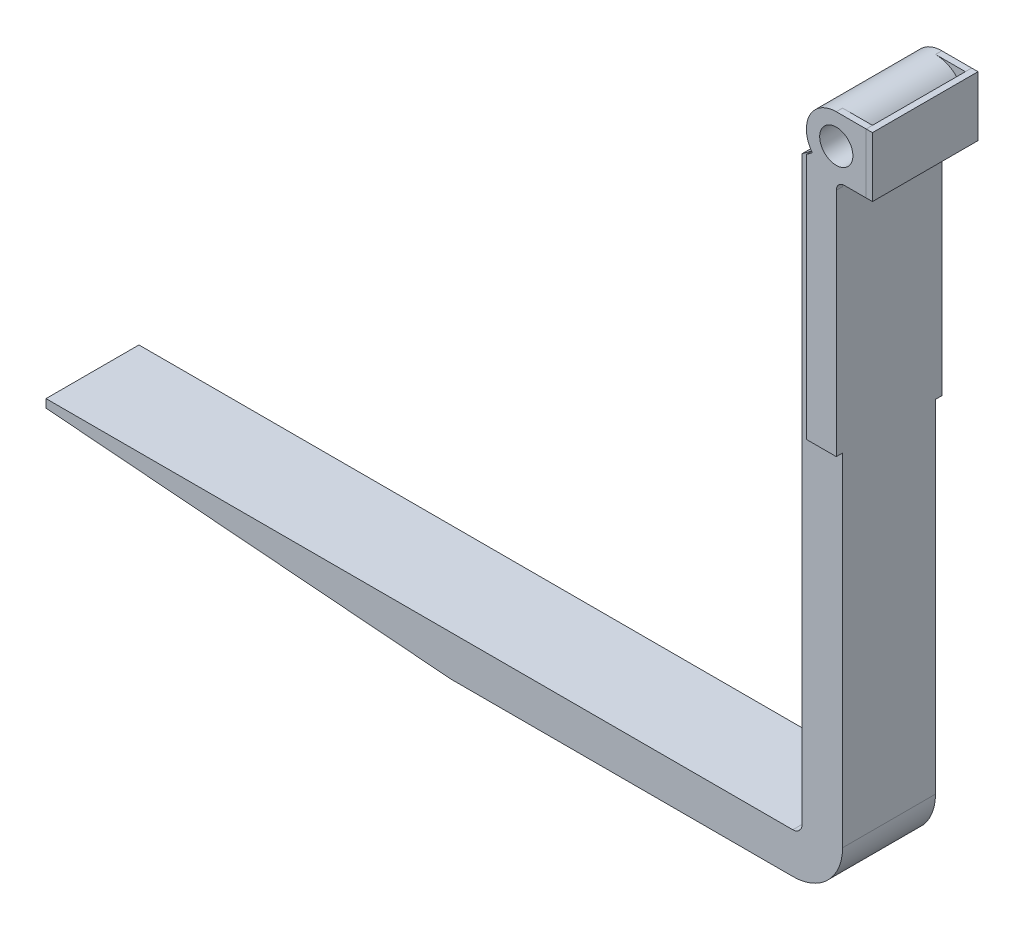
ISO-10303-21;
HEADER;
FILE_DESCRIPTION(('STEP AP214'),'2;1');
FILE_NAME('part.step','',(''),(''),'','','');
FILE_SCHEMA(('AUTOMOTIVE_DESIGN { 1 0 10303 214 1 1 1 1 }'));
ENDSEC;
DATA;
#1=APPLICATION_CONTEXT('core data for automotive mechanical design processes');
#2=APPLICATION_PROTOCOL_DEFINITION('international standard','automotive_design',2000,#1);
#3=PRODUCT_CONTEXT('',#1,'mechanical');
#4=PRODUCT('Part','Part','',(#3));
#5=PRODUCT_RELATED_PRODUCT_CATEGORY('part','',(#4));
#6=PRODUCT_DEFINITION_FORMATION('','',#4);
#7=PRODUCT_DEFINITION_CONTEXT('part definition',#1,'design');
#8=PRODUCT_DEFINITION('design','',#6,#7);
#9=PRODUCT_DEFINITION_SHAPE('','',#8);
#10=(LENGTH_UNIT() NAMED_UNIT(*) SI_UNIT(.MILLI.,.METRE.));
#11=(NAMED_UNIT(*) PLANE_ANGLE_UNIT() SI_UNIT($,.RADIAN.));
#12=(NAMED_UNIT(*) SI_UNIT($,.STERADIAN.) SOLID_ANGLE_UNIT());
#13=UNCERTAINTY_MEASURE_WITH_UNIT(LENGTH_MEASURE(1.E-05),#10,'distance_accuracy_value','');
#14=(GEOMETRIC_REPRESENTATION_CONTEXT(3) GLOBAL_UNCERTAINTY_ASSIGNED_CONTEXT((#13)) GLOBAL_UNIT_ASSIGNED_CONTEXT((#10,
#11,#12)) REPRESENTATION_CONTEXT('',''));
#15=CARTESIAN_POINT('',(0.,0.,0.));
#16=DIRECTION('',(0.,0.,1.));
#17=DIRECTION('',(1.,0.,0.));
#18=AXIS2_PLACEMENT_3D('',#15,#16,#17);
#19=CARTESIAN_POINT('',(54.4999999999999,1040.,79.5));
#20=DIRECTION('',(0.,0.,-1.));
#21=DIRECTION('',(-1.,0.,0.));
#22=AXIS2_PLACEMENT_3D('',#19,#20,#21);
#23=PLANE('',#22);
#24=DIRECTION('',(0.,-1.,0.));
#25=VECTOR('',#24,1.);
#26=CARTESIAN_POINT('',(44.9999999999999,1040.,79.5));
#27=LINE('',#26,#25);
#28=CARTESIAN_POINT('',(44.9999999999999,1040.,79.5));
#29=VERTEX_POINT('',#28);
#30=CARTESIAN_POINT('',(45.,950.,79.5));
#31=VERTEX_POINT('',#30);
#32=EDGE_CURVE('E118',#29,#31,#27,.T.);
#33=ORIENTED_EDGE('',*,*,#32,.T.);
#34=DIRECTION('',(-1.,0.,0.));
#35=VECTOR('',#34,1.);
#36=CARTESIAN_POINT('',(54.5,950.,79.5));
#37=LINE('',#36,#35);
#38=CARTESIAN_POINT('',(54.5,950.,79.5));
#39=VERTEX_POINT('',#38);
#40=EDGE_CURVE('E13',#39,#31,#37,.T.);
#41=ORIENTED_EDGE('',*,*,#40,.F.);
#42=DIRECTION('',(0.,-1.,0.));
#43=VECTOR('',#42,1.);
#44=CARTESIAN_POINT('',(54.4999999999999,1040.,79.5));
#45=LINE('',#44,#43);
#46=CARTESIAN_POINT('',(54.4999999999999,1040.,79.5));
#47=VERTEX_POINT('',#46);
#48=EDGE_CURVE('E107',#47,#39,#45,.T.);
#49=ORIENTED_EDGE('',*,*,#48,.F.);
#50=DIRECTION('',(-1.,0.,0.));
#51=VECTOR('',#50,1.);
#52=CARTESIAN_POINT('',(54.4999999999999,1040.,79.5));
#53=LINE('',#52,#51);
#54=EDGE_CURVE('E117',#47,#29,#53,.T.);
#55=ORIENTED_EDGE('',*,*,#54,.T.);
#56=EDGE_LOOP('',(#33,#41,#49,#55));
#57=FACE_BOUND('',#56,.T.);
#58=ADVANCED_FACE('F60',(#57),#23,.F.);
#59=CARTESIAN_POINT('',(54.5,950.,79.5));
#60=DIRECTION('',(0.,1.,0.));
#61=DIRECTION('',(-1.,0.,0.));
#62=AXIS2_PLACEMENT_3D('',#59,#60,#61);
#63=PLANE('',#62);
#64=DIRECTION('',(0.,0.,-1.));
#65=VECTOR('',#64,1.);
#66=CARTESIAN_POINT('',(45.,950.,79.5));
#67=LINE('',#66,#65);
#68=CARTESIAN_POINT('',(45.,950.,-79.5));
#69=VERTEX_POINT('',#68);
#70=EDGE_CURVE('E115',#31,#69,#67,.T.);
#71=ORIENTED_EDGE('',*,*,#70,.T.);
#72=DIRECTION('',(-1.,0.,0.));
#73=VECTOR('',#72,1.);
#74=CARTESIAN_POINT('',(54.5,950.,-79.5));
#75=LINE('',#74,#73);
#76=CARTESIAN_POINT('',(54.5,950.,-79.5));
#77=VERTEX_POINT('',#76);
#78=EDGE_CURVE('E63',#77,#69,#75,.T.);
#79=ORIENTED_EDGE('',*,*,#78,.F.);
#80=DIRECTION('',(0.,0.,-1.));
#81=VECTOR('',#80,1.);
#82=CARTESIAN_POINT('',(54.5,950.,79.5));
#83=LINE('',#82,#81);
#84=EDGE_CURVE('E103',#39,#77,#83,.T.);
#85=ORIENTED_EDGE('',*,*,#84,.F.);
#86=ORIENTED_EDGE('',*,*,#40,.T.);
#87=EDGE_LOOP('',(#71,#79,#85,#86));
#88=FACE_BOUND('',#87,.T.);
#89=ADVANCED_FACE('F112',(#88),#63,.F.);
#90=CARTESIAN_POINT('',(54.4999999999999,1040.,-79.5));
#91=DIRECTION('',(0.,0.,1.));
#92=DIRECTION('',(1.,0.,0.));
#93=AXIS2_PLACEMENT_3D('',#90,#91,#92);
#94=PLANE('',#93);
#95=DIRECTION('',(0.,1.,0.));
#96=VECTOR('',#95,1.);
#97=CARTESIAN_POINT('',(44.9999999999999,1040.,-79.5));
#98=LINE('',#97,#96);
#99=CARTESIAN_POINT('',(44.9999999999999,1040.,-79.5));
#100=VERTEX_POINT('',#99);
#101=EDGE_CURVE('E89',#69,#100,#98,.T.);
#102=ORIENTED_EDGE('',*,*,#101,.T.);
#103=DIRECTION('',(-1.,0.,0.));
#104=VECTOR('',#103,1.);
#105=CARTESIAN_POINT('',(54.4999999999999,1040.,-79.5));
#106=LINE('',#105,#104);
#107=CARTESIAN_POINT('',(54.4999999999999,1040.,-79.5));
#108=VERTEX_POINT('',#107);
#109=EDGE_CURVE('E114',#108,#100,#106,.T.);
#110=ORIENTED_EDGE('',*,*,#109,.F.);
#111=DIRECTION('',(0.,1.,0.));
#112=VECTOR('',#111,1.);
#113=CARTESIAN_POINT('',(54.4999999999999,1040.,-79.5));
#114=LINE('',#113,#112);
#115=EDGE_CURVE('E106',#77,#108,#114,.T.);
#116=ORIENTED_EDGE('',*,*,#115,.F.);
#117=ORIENTED_EDGE('',*,*,#78,.T.);
#118=EDGE_LOOP('',(#102,#110,#116,#117));
#119=FACE_BOUND('',#118,.T.);
#120=ADVANCED_FACE('F111',(#119),#94,.F.);
#121=CARTESIAN_POINT('',(54.4999999999999,1040.,79.5));
#122=DIRECTION('',(0.,-1.,0.));
#123=DIRECTION('',(1.,0.,0.));
#124=AXIS2_PLACEMENT_3D('',#121,#122,#123);
#125=PLANE('',#124);
#126=DIRECTION('',(0.,0.,1.));
#127=VECTOR('',#126,1.);
#128=CARTESIAN_POINT('',(44.9999999999999,1040.,79.5));
#129=LINE('',#128,#127);
#130=EDGE_CURVE('E96',#100,#29,#129,.T.);
#131=ORIENTED_EDGE('',*,*,#130,.T.);
#132=ORIENTED_EDGE('',*,*,#54,.F.);
#133=DIRECTION('',(0.,0.,1.));
#134=VECTOR('',#133,1.);
#135=CARTESIAN_POINT('',(54.4999999999999,1040.,79.5));
#136=LINE('',#135,#134);
#137=EDGE_CURVE('E71',#108,#47,#136,.T.);
#138=ORIENTED_EDGE('',*,*,#137,.F.);
#139=ORIENTED_EDGE('',*,*,#109,.T.);
#140=EDGE_LOOP('',(#131,#132,#138,#139));
#141=FACE_BOUND('',#140,.T.);
#142=ADVANCED_FACE('F130',(#141),#125,.F.);
#143=CARTESIAN_POINT('',(54.5000000000001,0.,0.));
#144=DIRECTION('',(1.,0.,0.));
#145=DIRECTION('',(0.,1.,0.));
#146=AXIS2_PLACEMENT_3D('',#143,#144,#145);
#147=PLANE('',#146);
#148=ORIENTED_EDGE('',*,*,#48,.T.);
#149=ORIENTED_EDGE('',*,*,#84,.T.);
#150=ORIENTED_EDGE('',*,*,#115,.T.);
#151=ORIENTED_EDGE('',*,*,#137,.T.);
#152=EDGE_LOOP('',(#148,#149,#150,#151));
#153=FACE_BOUND('',#152,.T.);
#154=ADVANCED_FACE('F102',(#153),#147,.T.);
#155=CARTESIAN_POINT('',(45.0000000000001,0.,0.));
#156=DIRECTION('',(1.,0.,0.));
#157=DIRECTION('',(0.,1.,0.));
#158=AXIS2_PLACEMENT_3D('',#155,#156,#157);
#159=PLANE('',#158);
#160=ORIENTED_EDGE('',*,*,#32,.F.);
#161=ORIENTED_EDGE('',*,*,#130,.F.);
#162=ORIENTED_EDGE('',*,*,#101,.F.);
#163=ORIENTED_EDGE('',*,*,#70,.F.);
#164=EDGE_LOOP('',(#160,#161,#162,#163));
#165=FACE_BOUND('',#164,.T.);
#166=ADVANCED_FACE('F128',(#165),#159,.F.);
#167=CLOSED_SHELL('',(#58,#89,#120,#142,#154,#166));
#168=MANIFOLD_SOLID_BREP('B2',#167);
#169=CARTESIAN_POINT('',(-75.,75.,-70.));
#170=DIRECTION('',(0.,0.,-1.));
#171=DIRECTION('',(-1.,0.,0.));
#172=AXIS2_PLACEMENT_3D('',#169,#170,#171);
#173=PLANE('',#172);
#174=DIRECTION('',(0.804724130284083,0.593648948570219,0.));
#175=VECTOR('',#174,1.);
#176=CARTESIAN_POINT('',(-475.335015663069,644.343021232165,-70.));
#177=LINE('',#176,#175);
#178=CARTESIAN_POINT('',(-61.,950.,-70.));
#179=VERTEX_POINT('',#178);
#180=CARTESIAN_POINT('',(-45.,961.803278688525,-70.));
#181=VERTEX_POINT('',#180);
#182=EDGE_CURVE('E469',#179,#181,#177,.T.);
#183=ORIENTED_EDGE('',*,*,#182,.T.);
#184=DIRECTION('',(0.,-1.,0.));
#185=VECTOR('',#184,1.);
#186=CARTESIAN_POINT('',(-44.9999999999999,0.,-70.));
#187=LINE('',#186,#185);
#188=CARTESIAN_POINT('',(-45.,590.,-70.));
#189=VERTEX_POINT('',#188);
#190=EDGE_CURVE('E565',#181,#189,#187,.T.);
#191=ORIENTED_EDGE('',*,*,#190,.T.);
#192=DIRECTION('',(-1.,0.,0.));
#193=VECTOR('',#192,1.);
#194=CARTESIAN_POINT('',(0.,590.,-70.));
#195=LINE('',#194,#193);
#196=CARTESIAN_POINT('',(0.,590.,-70.));
#197=VERTEX_POINT('',#196);
#198=EDGE_CURVE('E198',#197,#189,#195,.T.);
#199=ORIENTED_EDGE('',*,*,#198,.F.);
#200=DIRECTION('',(0.,-1.,0.));
#201=VECTOR('',#200,1.);
#202=CARTESIAN_POINT('',(0.,950.,-70.));
#203=LINE('',#202,#201);
#204=CARTESIAN_POINT('',(0.,75.0000000000005,-70.));
#205=VERTEX_POINT('',#204);
#206=EDGE_CURVE('E514',#197,#205,#203,.T.);
#207=ORIENTED_EDGE('',*,*,#206,.T.);
#208=CARTESIAN_POINT('',(-75.,75.,-70.));
#209=DIRECTION('',(0.,0.,-1.));
#210=DIRECTION('',(-1.,0.,0.));
#211=AXIS2_PLACEMENT_3D('',#208,#209,#210);
#212=CIRCLE('',#211,75.);
#213=CARTESIAN_POINT('',(-75.0000000000005,0.,-70.));
#214=VERTEX_POINT('',#213);
#215=EDGE_CURVE('E512',#205,#214,#212,.T.);
#216=ORIENTED_EDGE('',*,*,#215,.T.);
#217=DIRECTION('',(-1.,0.,0.));
#218=VECTOR('',#217,1.);
#219=CARTESIAN_POINT('',(-75.0000000000005,0.,-70.));
#220=LINE('',#219,#218);
#221=CARTESIAN_POINT('',(-590.,0.,-69.9999999999998));
#222=VERTEX_POINT('',#221);
#223=EDGE_CURVE('E508',#214,#222,#220,.T.);
#224=ORIENTED_EDGE('',*,*,#223,.T.);
#225=DIRECTION('',(0.996854130580606,-0.0792580743166547,0.));
#226=VECTOR('',#225,1.);
#227=CARTESIAN_POINT('',(-84.1608042146896,-40.2183622878485,-70.));
#228=LINE('',#227,#226);
#229=CARTESIAN_POINT('',(-1200.,48.4999999999999,-70.));
#230=VERTEX_POINT('',#229);
#231=EDGE_CURVE('E54',#230,#222,#228,.T.);
#232=ORIENTED_EDGE('',*,*,#231,.F.);
#233=DIRECTION('',(0.,1.,0.));
#234=VECTOR('',#233,1.);
#235=CARTESIAN_POINT('',(-1200.,0.,-70.));
#236=LINE('',#235,#234);
#237=CARTESIAN_POINT('',(-1200.,61.,-70.));
#238=VERTEX_POINT('',#237);
#239=EDGE_CURVE('E506',#230,#238,#236,.T.);
#240=ORIENTED_EDGE('',*,*,#239,.T.);
#241=DIRECTION('',(1.,0.,0.));
#242=VECTOR('',#241,1.);
#243=CARTESIAN_POINT('',(-75.0000000000005,61.,-70.));
#244=LINE('',#243,#242);
#245=CARTESIAN_POINT('',(-75.0000000000005,61.,-70.));
#246=VERTEX_POINT('',#245);
#247=EDGE_CURVE('E482',#246,#238,#244,.F.);
#248=ORIENTED_EDGE('',*,*,#247,.F.);
#249=CARTESIAN_POINT('',(-75.,75.,-70.));
#250=DIRECTION('',(0.,0.,1.));
#251=DIRECTION('',(1.,0.,0.));
#252=AXIS2_PLACEMENT_3D('',#249,#250,#251);
#253=CIRCLE('',#252,14.);
#254=CARTESIAN_POINT('',(-61.,75.0000000000001,-70.));
#255=VERTEX_POINT('',#254);
#256=EDGE_CURVE('E487',#255,#246,#253,.F.);
#257=ORIENTED_EDGE('',*,*,#256,.F.);
#258=DIRECTION('',(0.,-1.,0.));
#259=VECTOR('',#258,1.);
#260=CARTESIAN_POINT('',(-61.,950.,-70.));
#261=LINE('',#260,#259);
#262=EDGE_CURVE('E517',#179,#255,#261,.T.);
#263=ORIENTED_EDGE('',*,*,#262,.F.);
#264=EDGE_LOOP('',(#183,#191,#199,#207,#216,#224,#232,#240,#248,#257,#263));
#265=FACE_BOUND('',#264,.T.);
#266=ADVANCED_FACE('F182',(#265),#173,.T.);
#267=CARTESIAN_POINT('',(-75.0000000000005,0.,70.));
#268=DIRECTION('',(0.,-1.,0.));
#269=DIRECTION('',(0.,0.,-1.));
#270=AXIS2_PLACEMENT_3D('',#267,#268,#269);
#271=PLANE('',#270);
#272=DIRECTION('',(-1.,0.,0.));
#273=VECTOR('',#272,1.);
#274=CARTESIAN_POINT('',(-75.0000000000005,0.,70.));
#275=LINE('',#274,#273);
#276=CARTESIAN_POINT('',(-75.0000000000005,0.,70.));
#277=VERTEX_POINT('',#276);
#278=CARTESIAN_POINT('',(-590.,0.,70.));
#279=VERTEX_POINT('',#278);
#280=EDGE_CURVE('E491',#277,#279,#275,.T.);
#281=ORIENTED_EDGE('',*,*,#280,.T.);
#282=DIRECTION('',(0.,0.,-1.));
#283=VECTOR('',#282,1.);
#284=CARTESIAN_POINT('',(-590.,0.,2166.14061172003));
#285=LINE('',#284,#283);
#286=EDGE_CURVE('E480',#279,#222,#285,.T.);
#287=ORIENTED_EDGE('',*,*,#286,.T.);
#288=ORIENTED_EDGE('',*,*,#223,.F.);
#289=DIRECTION('',(0.,0.,-1.));
#290=VECTOR('',#289,1.);
#291=CARTESIAN_POINT('',(-75.0000000000005,0.,70.));
#292=LINE('',#291,#290);
#293=EDGE_CURVE('E535',#277,#214,#292,.T.);
#294=ORIENTED_EDGE('',*,*,#293,.F.);
#295=EDGE_LOOP('',(#281,#287,#288,#294));
#296=FACE_BOUND('',#295,.T.);
#297=ADVANCED_FACE('F630',(#296),#271,.T.);
#298=CARTESIAN_POINT('',(-75.0000000000005,61.,70.));
#299=DIRECTION('',(0.,-1.,0.));
#300=DIRECTION('',(0.,0.,-1.));
#301=AXIS2_PLACEMENT_3D('',#298,#299,#300);
#302=PLANE('',#301);
#303=ORIENTED_EDGE('',*,*,#247,.T.);
#304=DIRECTION('',(0.,0.,-1.));
#305=VECTOR('',#304,1.);
#306=CARTESIAN_POINT('',(-1200.,61.,70.));
#307=LINE('',#306,#305);
#308=CARTESIAN_POINT('',(-1200.,61.,70.));
#309=VERTEX_POINT('',#308);
#310=EDGE_CURVE('E186',#309,#238,#307,.T.);
#311=ORIENTED_EDGE('',*,*,#310,.F.);
#312=DIRECTION('',(1.,0.,0.));
#313=VECTOR('',#312,1.);
#314=CARTESIAN_POINT('',(-75.0000000000005,61.,70.));
#315=LINE('',#314,#313);
#316=CARTESIAN_POINT('',(-75.0000000000005,61.,70.));
#317=VERTEX_POINT('',#316);
#318=EDGE_CURVE('E484',#317,#309,#315,.F.);
#319=ORIENTED_EDGE('',*,*,#318,.F.);
#320=DIRECTION('',(0.,0.,-1.));
#321=VECTOR('',#320,1.);
#322=CARTESIAN_POINT('',(-75.0000000000005,61.,70.));
#323=LINE('',#322,#321);
#324=EDGE_CURVE('E501',#317,#246,#323,.T.);
#325=ORIENTED_EDGE('',*,*,#324,.T.);
#326=EDGE_LOOP('',(#303,#311,#319,#325));
#327=FACE_BOUND('',#326,.T.);
#328=ADVANCED_FACE('F181',(#327),#302,.F.);
#329=CARTESIAN_POINT('',(-1200.,0.,70.));
#330=DIRECTION('',(-1.,0.,0.));
#331=DIRECTION('',(0.,-1.,0.));
#332=AXIS2_PLACEMENT_3D('',#329,#330,#331);
#333=PLANE('',#332);
#334=DIRECTION('',(0.,0.,-1.));
#335=VECTOR('',#334,1.);
#336=CARTESIAN_POINT('',(-1200.,48.5,2166.14061172003));
#337=LINE('',#336,#335);
#338=CARTESIAN_POINT('',(-1200.,48.4999999999999,70.));
#339=VERTEX_POINT('',#338);
#340=EDGE_CURVE('E478',#339,#230,#337,.T.);
#341=ORIENTED_EDGE('',*,*,#340,.F.);
#342=DIRECTION('',(0.,1.,0.));
#343=VECTOR('',#342,1.);
#344=CARTESIAN_POINT('',(-1200.,0.,70.));
#345=LINE('',#344,#343);
#346=EDGE_CURVE('E488',#339,#309,#345,.T.);
#347=ORIENTED_EDGE('',*,*,#346,.T.);
#348=ORIENTED_EDGE('',*,*,#310,.T.);
#349=ORIENTED_EDGE('',*,*,#239,.F.);
#350=EDGE_LOOP('',(#341,#347,#348,#349));
#351=FACE_BOUND('',#350,.T.);
#352=ADVANCED_FACE('F540',(#351),#333,.T.);
#353=CARTESIAN_POINT('',(-75.,75.,70.));
#354=DIRECTION('',(0.,0.,-1.));
#355=DIRECTION('',(-1.,0.,0.));
#356=AXIS2_PLACEMENT_3D('',#353,#354,#355);
#357=CYLINDRICAL_SURFACE('',#356,75.);
#358=ORIENTED_EDGE('',*,*,#215,.F.);
#359=DIRECTION('',(0.,0.,-1.));
#360=VECTOR('',#359,1.);
#361=CARTESIAN_POINT('',(0.,75.0000000000005,70.));
#362=LINE('',#361,#360);
#363=CARTESIAN_POINT('',(0.,75.0000000000005,70.));
#364=VERTEX_POINT('',#363);
#365=EDGE_CURVE('E530',#364,#205,#362,.T.);
#366=ORIENTED_EDGE('',*,*,#365,.F.);
#367=CARTESIAN_POINT('',(-75.,75.,70.));
#368=DIRECTION('',(0.,0.,-1.));
#369=DIRECTION('',(-1.,0.,0.));
#370=AXIS2_PLACEMENT_3D('',#367,#368,#369);
#371=CIRCLE('',#370,75.);
#372=EDGE_CURVE('E493',#364,#277,#371,.T.);
#373=ORIENTED_EDGE('',*,*,#372,.T.);
#374=ORIENTED_EDGE('',*,*,#293,.T.);
#375=EDGE_LOOP('',(#358,#366,#373,#374));
#376=FACE_BOUND('',#375,.T.);
#377=ADVANCED_FACE('F623',(#376),#357,.T.);
#378=CARTESIAN_POINT('',(0.,950.,70.));
#379=DIRECTION('',(1.,0.,0.));
#380=DIRECTION('',(0.,1.,0.));
#381=AXIS2_PLACEMENT_3D('',#378,#379,#380);
#382=PLANE('',#381);
#383=CARTESIAN_POINT('',(0.,950.,-70.));
#384=VERTEX_POINT('',#383);
#385=CARTESIAN_POINT('',(0.,937.5,-70.));
#386=VERTEX_POINT('',#385);
#387=EDGE_CURVE('E204',#384,#386,#203,.T.);
#388=ORIENTED_EDGE('',*,*,#387,.F.);
#389=DIRECTION('',(0.,0.,-1.));
#390=VECTOR('',#389,1.);
#391=CARTESIAN_POINT('',(0.,950.,70.));
#392=LINE('',#391,#390);
#393=CARTESIAN_POINT('',(0.,950.,70.));
#394=VERTEX_POINT('',#393);
#395=EDGE_CURVE('E527',#394,#384,#392,.T.);
#396=ORIENTED_EDGE('',*,*,#395,.F.);
#397=DIRECTION('',(0.,-1.,0.));
#398=VECTOR('',#397,1.);
#399=CARTESIAN_POINT('',(0.,950.,70.));
#400=LINE('',#399,#398);
#401=CARTESIAN_POINT('',(0.,937.5,70.));
#402=VERTEX_POINT('',#401);
#403=EDGE_CURVE('E499',#394,#402,#400,.T.);
#404=ORIENTED_EDGE('',*,*,#403,.T.);
#405=DIRECTION('',(0.,0.,-1.));
#406=VECTOR('',#405,1.);
#407=CARTESIAN_POINT('',(0.,937.5,79.5));
#408=LINE('',#407,#406);
#409=CARTESIAN_POINT('',(0.,937.5,79.5));
#410=VERTEX_POINT('',#409);
#411=EDGE_CURVE('E443',#410,#402,#408,.T.);
#412=ORIENTED_EDGE('',*,*,#411,.F.);
#413=DIRECTION('',(0.,1.,0.));
#414=VECTOR('',#413,1.);
#415=CARTESIAN_POINT('',(0.,0.,79.5));
#416=LINE('',#415,#414);
#417=CARTESIAN_POINT('',(0.,590.,79.5));
#418=VERTEX_POINT('',#417);
#419=EDGE_CURVE('E418',#418,#410,#416,.T.);
#420=ORIENTED_EDGE('',*,*,#419,.F.);
#421=DIRECTION('',(0.,0.,-1.));
#422=VECTOR('',#421,1.);
#423=CARTESIAN_POINT('',(0.,590.,79.5));
#424=LINE('',#423,#422);
#425=CARTESIAN_POINT('',(0.,590.,70.));
#426=VERTEX_POINT('',#425);
#427=EDGE_CURVE('E450',#418,#426,#424,.T.);
#428=ORIENTED_EDGE('',*,*,#427,.T.);
#429=EDGE_CURVE('E500',#426,#364,#400,.T.);
#430=ORIENTED_EDGE('',*,*,#429,.T.);
#431=ORIENTED_EDGE('',*,*,#365,.T.);
#432=ORIENTED_EDGE('',*,*,#206,.F.);
#433=DIRECTION('',(0.,0.,1.));
#434=VECTOR('',#433,1.);
#435=CARTESIAN_POINT('',(0.,590.,-79.5));
#436=LINE('',#435,#434);
#437=CARTESIAN_POINT('',(0.,590.,-79.5));
#438=VERTEX_POINT('',#437);
#439=EDGE_CURVE('E591',#438,#197,#436,.T.);
#440=ORIENTED_EDGE('',*,*,#439,.F.);
#441=DIRECTION('',(0.,1.,0.));
#442=VECTOR('',#441,1.);
#443=CARTESIAN_POINT('',(0.,0.,-79.5));
#444=LINE('',#443,#442);
#445=CARTESIAN_POINT('',(0.,937.5,-79.5));
#446=VERTEX_POINT('',#445);
#447=EDGE_CURVE('E597',#438,#446,#444,.T.);
#448=ORIENTED_EDGE('',*,*,#447,.T.);
#449=DIRECTION('',(0.,0.,1.));
#450=VECTOR('',#449,1.);
#451=CARTESIAN_POINT('',(0.,937.5,-79.5));
#452=LINE('',#451,#450);
#453=EDGE_CURVE('E393',#446,#386,#452,.T.);
#454=ORIENTED_EDGE('',*,*,#453,.T.);
#455=EDGE_LOOP('',(#388,#396,#404,#412,#420,#428,#430,#431,#432,#440,#448,#454));
#456=FACE_BOUND('',#455,.T.);
#457=ADVANCED_FACE('F596',(#456),#382,.T.);
#458=CARTESIAN_POINT('',(-61.,950.,70.));
#459=DIRECTION('',(1.,0.,0.));
#460=DIRECTION('',(0.,1.,0.));
#461=AXIS2_PLACEMENT_3D('',#458,#459,#460);
#462=PLANE('',#461);
#463=ORIENTED_EDGE('',*,*,#262,.T.);
#464=DIRECTION('',(0.,0.,-1.));
#465=VECTOR('',#464,1.);
#466=CARTESIAN_POINT('',(-61.,75.0000000000001,70.));
#467=LINE('',#466,#465);
#468=CARTESIAN_POINT('',(-61.,75.0000000000001,70.));
#469=VERTEX_POINT('',#468);
#470=EDGE_CURVE('E524',#469,#255,#467,.T.);
#471=ORIENTED_EDGE('',*,*,#470,.F.);
#472=DIRECTION('',(0.,-1.,0.));
#473=VECTOR('',#472,1.);
#474=CARTESIAN_POINT('',(-61.,950.,70.));
#475=LINE('',#474,#473);
#476=CARTESIAN_POINT('',(-61.,950.,70.));
#477=VERTEX_POINT('',#476);
#478=EDGE_CURVE('E498',#477,#469,#475,.T.);
#479=ORIENTED_EDGE('',*,*,#478,.F.);
#480=DIRECTION('',(0.,0.,-1.));
#481=VECTOR('',#480,1.);
#482=CARTESIAN_POINT('',(-61.,950.,70.));
#483=LINE('',#482,#481);
#484=EDGE_CURVE('E523',#477,#179,#483,.T.);
#485=ORIENTED_EDGE('',*,*,#484,.T.);
#486=EDGE_LOOP('',(#463,#471,#479,#485));
#487=FACE_BOUND('',#486,.T.);
#488=ADVANCED_FACE('F558',(#487),#462,.F.);
#489=CARTESIAN_POINT('',(-75.,75.,70.));
#490=DIRECTION('',(0.,0.,-1.));
#491=DIRECTION('',(-1.,0.,0.));
#492=AXIS2_PLACEMENT_3D('',#489,#490,#491);
#493=CYLINDRICAL_SURFACE('',#492,14.);
#494=ORIENTED_EDGE('',*,*,#256,.T.);
#495=ORIENTED_EDGE('',*,*,#324,.F.);
#496=CARTESIAN_POINT('',(-75.,75.,70.));
#497=DIRECTION('',(0.,0.,1.));
#498=DIRECTION('',(1.,0.,0.));
#499=AXIS2_PLACEMENT_3D('',#496,#497,#498);
#500=CIRCLE('',#499,14.);
#501=EDGE_CURVE('E504',#469,#317,#500,.F.);
#502=ORIENTED_EDGE('',*,*,#501,.F.);
#503=ORIENTED_EDGE('',*,*,#470,.T.);
#504=EDGE_LOOP('',(#494,#495,#502,#503));
#505=FACE_BOUND('',#504,.T.);
#506=ADVANCED_FACE('F560',(#505),#493,.F.);
#507=CARTESIAN_POINT('',(-75.,75.,70.));
#508=DIRECTION('',(0.,0.,-1.));
#509=DIRECTION('',(-1.,0.,0.));
#510=AXIS2_PLACEMENT_3D('',#507,#508,#509);
#511=PLANE('',#510);
#512=ORIENTED_EDGE('',*,*,#429,.F.);
#513=DIRECTION('',(-1.,0.,0.));
#514=VECTOR('',#513,1.);
#515=CARTESIAN_POINT('',(0.,590.,70.));
#516=LINE('',#515,#514);
#517=CARTESIAN_POINT('',(-45.,590.,70.));
#518=VERTEX_POINT('',#517);
#519=EDGE_CURVE('E432',#426,#518,#516,.T.);
#520=ORIENTED_EDGE('',*,*,#519,.T.);
#521=DIRECTION('',(0.,-1.,0.));
#522=VECTOR('',#521,1.);
#523=CARTESIAN_POINT('',(-44.9999999999999,0.,70.));
#524=LINE('',#523,#522);
#525=CARTESIAN_POINT('',(-45.,961.803278688525,70.));
#526=VERTEX_POINT('',#525);
#527=EDGE_CURVE('E431',#526,#518,#524,.T.);
#528=ORIENTED_EDGE('',*,*,#527,.F.);
#529=DIRECTION('',(0.804724130284083,0.593648948570219,0.));
#530=VECTOR('',#529,1.);
#531=CARTESIAN_POINT('',(-475.335015663069,644.343021232165,70.));
#532=LINE('',#531,#530);
#533=EDGE_CURVE('E467',#477,#526,#532,.T.);
#534=ORIENTED_EDGE('',*,*,#533,.F.);
#535=ORIENTED_EDGE('',*,*,#478,.T.);
#536=ORIENTED_EDGE('',*,*,#501,.T.);
#537=ORIENTED_EDGE('',*,*,#318,.T.);
#538=ORIENTED_EDGE('',*,*,#346,.F.);
#539=DIRECTION('',(0.996854130580606,-0.0792580743166547,0.));
#540=VECTOR('',#539,1.);
#541=CARTESIAN_POINT('',(-84.1608042146896,-40.2183622878485,70.));
#542=LINE('',#541,#540);
#543=EDGE_CURVE('E477',#339,#279,#542,.T.);
#544=ORIENTED_EDGE('',*,*,#543,.T.);
#545=ORIENTED_EDGE('',*,*,#280,.F.);
#546=ORIENTED_EDGE('',*,*,#372,.F.);
#547=EDGE_LOOP('',(#512,#520,#528,#534,#535,#536,#537,#538,#544,#545,#546));
#548=FACE_BOUND('',#547,.T.);
#549=ADVANCED_FACE('F552',(#548),#511,.F.);
#550=CARTESIAN_POINT('',(-1200.,48.5,2166.14061172003));
#551=DIRECTION('',(0.0792580743166547,0.996854130580606,0.));
#552=DIRECTION('',(-0.996854130580606,0.0792580743166547,0.));
#553=AXIS2_PLACEMENT_3D('',#550,#551,#552);
#554=PLANE('',#553);
#555=ORIENTED_EDGE('',*,*,#543,.F.);
#556=ORIENTED_EDGE('',*,*,#340,.T.);
#557=ORIENTED_EDGE('',*,*,#231,.T.);
#558=ORIENTED_EDGE('',*,*,#286,.F.);
#559=EDGE_LOOP('',(#555,#556,#557,#558));
#560=FACE_BOUND('',#559,.T.);
#561=ADVANCED_FACE('F548',(#560),#554,.F.);
#562=CARTESIAN_POINT('',(-475.335015663069,644.343021232165,70.));
#563=DIRECTION('',(-0.593648948570219,0.804724130284083,0.));
#564=DIRECTION('',(-0.804724130284083,-0.593648948570219,0.));
#565=AXIS2_PLACEMENT_3D('',#562,#563,#564);
#566=PLANE('',#565);
#567=ORIENTED_EDGE('',*,*,#182,.F.);
#568=ORIENTED_EDGE('',*,*,#484,.F.);
#569=ORIENTED_EDGE('',*,*,#533,.T.);
#570=DIRECTION('',(0.,0.,-1.));
#571=VECTOR('',#570,1.);
#572=CARTESIAN_POINT('',(-45.,961.803278688525,79.5));
#573=LINE('',#572,#571);
#574=CARTESIAN_POINT('',(-45.,961.803278688525,79.5));
#575=VERTEX_POINT('',#574);
#576=EDGE_CURVE('E453',#575,#526,#573,.T.);
#577=ORIENTED_EDGE('',*,*,#576,.F.);
#578=DIRECTION('',(-0.804724130284083,-0.593648948570219,0.));
#579=VECTOR('',#578,1.);
#580=CARTESIAN_POINT('',(-475.335015663069,644.343021232166,79.5));
#581=LINE('',#580,#579);
#582=CARTESIAN_POINT('',(-36.2125858627837,968.28579731434,79.5));
#583=VERTEX_POINT('',#582);
#584=EDGE_CURVE('E406',#583,#575,#581,.T.);
#585=ORIENTED_EDGE('',*,*,#584,.F.);
#586=DIRECTION('',(0.,0.,-1.));
#587=VECTOR('',#586,1.);
#588=CARTESIAN_POINT('',(-36.2125858627836,968.28579731434,70.));
#589=LINE('',#588,#587);
#590=CARTESIAN_POINT('',(-36.2125858627837,968.28579731434,-79.5));
#591=VERTEX_POINT('',#590);
#592=EDGE_CURVE('E471',#583,#591,#589,.T.);
#593=ORIENTED_EDGE('',*,*,#592,.T.);
#594=DIRECTION('',(-0.804724130284083,-0.593648948570219,0.));
#595=VECTOR('',#594,1.);
#596=CARTESIAN_POINT('',(-475.335015663069,644.343021232166,-79.5));
#597=LINE('',#596,#595);
#598=CARTESIAN_POINT('',(-45.,961.803278688525,-79.5));
#599=VERTEX_POINT('',#598);
#600=EDGE_CURVE('E568',#591,#599,#597,.T.);
#601=ORIENTED_EDGE('',*,*,#600,.T.);
#602=DIRECTION('',(0.,0.,1.));
#603=VECTOR('',#602,1.);
#604=CARTESIAN_POINT('',(-45.,961.803278688525,-79.5));
#605=LINE('',#604,#603);
#606=EDGE_CURVE('E570',#599,#181,#605,.T.);
#607=ORIENTED_EDGE('',*,*,#606,.T.);
#608=EDGE_LOOP('',(#567,#568,#569,#577,#585,#593,#601,#607));
#609=FACE_BOUND('',#608,.T.);
#610=ADVANCED_FACE('F566',(#609),#566,.T.);
#611=CARTESIAN_POINT('',(0.,995.,70.));
#612=DIRECTION('',(0.,0.,-1.));
#613=DIRECTION('',(-1.,0.,0.));
#614=AXIS2_PLACEMENT_3D('',#611,#612,#613);
#615=CYLINDRICAL_SURFACE('',#614,45.);
#616=ORIENTED_EDGE('',*,*,#395,.T.);
#617=CARTESIAN_POINT('',(0.,995.,-70.));
#618=DIRECTION('',(0.,0.,1.));
#619=DIRECTION('',(1.,0.,0.));
#620=AXIS2_PLACEMENT_3D('',#617,#618,#619);
#621=CIRCLE('',#620,45.);
#622=CARTESIAN_POINT('',(45.,995.,-70.));
#623=VERTEX_POINT('',#622);
#624=EDGE_CURVE('E470',#384,#623,#621,.T.);
#625=ORIENTED_EDGE('',*,*,#624,.T.);
#626=CARTESIAN_POINT('',(0.,1040.,-70.));
#627=VERTEX_POINT('',#626);
#628=EDGE_CURVE('E464',#623,#627,#621,.T.);
#629=ORIENTED_EDGE('',*,*,#628,.T.);
#630=DIRECTION('',(0.,0.,1.));
#631=VECTOR('',#630,1.);
#632=CARTESIAN_POINT('',(0.,1040.,-79.5));
#633=LINE('',#632,#631);
#634=CARTESIAN_POINT('',(0.,1040.,-79.5));
#635=VERTEX_POINT('',#634);
#636=EDGE_CURVE('E573',#635,#627,#633,.T.);
#637=ORIENTED_EDGE('',*,*,#636,.F.);
#638=CARTESIAN_POINT('',(0.,995.,-79.5));
#639=DIRECTION('',(0.,0.,1.));
#640=DIRECTION('',(1.,0.,0.));
#641=AXIS2_PLACEMENT_3D('',#638,#639,#640);
#642=CIRCLE('',#641,45.);
#643=EDGE_CURVE('E608',#635,#591,#642,.T.);
#644=ORIENTED_EDGE('',*,*,#643,.T.);
#645=ORIENTED_EDGE('',*,*,#592,.F.);
#646=CARTESIAN_POINT('',(0.,995.,79.5));
#647=DIRECTION('',(0.,0.,1.));
#648=DIRECTION('',(1.,0.,0.));
#649=AXIS2_PLACEMENT_3D('',#646,#647,#648);
#650=CIRCLE('',#649,45.);
#651=CARTESIAN_POINT('',(0.,1040.,79.5));
#652=VERTEX_POINT('',#651);
#653=EDGE_CURVE('E407',#652,#583,#650,.T.);
#654=ORIENTED_EDGE('',*,*,#653,.F.);
#655=DIRECTION('',(0.,0.,-1.));
#656=VECTOR('',#655,1.);
#657=CARTESIAN_POINT('',(0.,1040.,79.5));
#658=LINE('',#657,#656);
#659=CARTESIAN_POINT('',(0.,1040.,70.));
#660=VERTEX_POINT('',#659);
#661=EDGE_CURVE('E460',#652,#660,#658,.T.);
#662=ORIENTED_EDGE('',*,*,#661,.T.);
#663=CARTESIAN_POINT('',(0.,995.,70.));
#664=DIRECTION('',(0.,0.,1.));
#665=DIRECTION('',(1.,0.,0.));
#666=AXIS2_PLACEMENT_3D('',#663,#664,#665);
#667=CIRCLE('',#666,45.);
#668=CARTESIAN_POINT('',(45.,995.,70.));
#669=VERTEX_POINT('',#668);
#670=EDGE_CURVE('E466',#669,#660,#667,.T.);
#671=ORIENTED_EDGE('',*,*,#670,.F.);
#672=EDGE_CURVE('E465',#394,#669,#667,.T.);
#673=ORIENTED_EDGE('',*,*,#672,.F.);
#674=EDGE_LOOP('',(#616,#625,#629,#637,#644,#645,#654,#662,#671,#673));
#675=FACE_BOUND('',#674,.T.);
#676=ADVANCED_FACE('F648',(#675),#615,.T.);
#677=CARTESIAN_POINT('',(0.,995.,70.));
#678=DIRECTION('',(0.,0.,-1.));
#679=DIRECTION('',(-1.,0.,0.));
#680=AXIS2_PLACEMENT_3D('',#677,#678,#679);
#681=CYLINDRICAL_SURFACE('',#680,25.);
#682=CARTESIAN_POINT('',(0.,995.,79.5));
#683=DIRECTION('',(0.,0.,1.));
#684=DIRECTION('',(1.,0.,0.));
#685=AXIS2_PLACEMENT_3D('',#682,#683,#684);
#686=CIRCLE('',#685,25.);
#687=CARTESIAN_POINT('',(25.,995.,79.5));
#688=VERTEX_POINT('',#687);
#689=EDGE_CURVE('E421',#688,#688,#686,.F.);
#690=ORIENTED_EDGE('',*,*,#689,.F.);
#691=EDGE_LOOP('',(#690));
#692=FACE_BOUND('',#691,.T.);
#693=CARTESIAN_POINT('',(0.,995.,-79.5));
#694=DIRECTION('',(0.,0.,1.));
#695=DIRECTION('',(1.,0.,0.));
#696=AXIS2_PLACEMENT_3D('',#693,#694,#695);
#697=CIRCLE('',#696,25.);
#698=CARTESIAN_POINT('',(25.,995.,-79.5));
#699=VERTEX_POINT('',#698);
#700=EDGE_CURVE('E590',#699,#699,#697,.F.);
#701=ORIENTED_EDGE('',*,*,#700,.T.);
#702=EDGE_LOOP('',(#701));
#703=FACE_BOUND('',#702,.T.);
#704=ADVANCED_FACE('F679',(#692,#703),#681,.F.);
#705=CARTESIAN_POINT('',(0.,0.,70.));
#706=DIRECTION('',(0.,0.,1.));
#707=DIRECTION('',(1.,0.,0.));
#708=AXIS2_PLACEMENT_3D('',#705,#706,#707);
#709=PLANE('',#708);
#710=DIRECTION('',(0.,-1.,0.));
#711=VECTOR('',#710,1.);
#712=CARTESIAN_POINT('',(45.0000000000001,0.,70.));
#713=LINE('',#712,#711);
#714=CARTESIAN_POINT('',(44.9999999999999,1040.,70.));
#715=VERTEX_POINT('',#714);
#716=EDGE_CURVE('E395',#715,#669,#713,.T.);
#717=ORIENTED_EDGE('',*,*,#716,.T.);
#718=ORIENTED_EDGE('',*,*,#670,.T.);
#719=DIRECTION('',(1.,0.,0.));
#720=VECTOR('',#719,1.);
#721=CARTESIAN_POINT('',(0.,1040.,70.));
#722=LINE('',#721,#720);
#723=EDGE_CURVE('E428',#660,#715,#722,.T.);
#724=ORIENTED_EDGE('',*,*,#723,.T.);
#725=EDGE_LOOP('',(#717,#718,#724));
#726=FACE_BOUND('',#725,.T.);
#727=ADVANCED_FACE('F680',(#726),#709,.F.);
#728=CARTESIAN_POINT('',(45.0000000000001,0.,79.5));
#729=DIRECTION('',(1.,0.,0.));
#730=DIRECTION('',(0.,1.,0.));
#731=AXIS2_PLACEMENT_3D('',#728,#729,#730);
#732=PLANE('',#731);
#733=ORIENTED_EDGE('',*,*,#716,.F.);
#734=DIRECTION('',(0.,0.,-1.));
#735=VECTOR('',#734,1.);
#736=CARTESIAN_POINT('',(44.9999999999999,1040.,79.5));
#737=LINE('',#736,#735);
#738=CARTESIAN_POINT('',(44.9999999999999,1040.,79.5));
#739=VERTEX_POINT('',#738);
#740=EDGE_CURVE('E458',#739,#715,#737,.T.);
#741=ORIENTED_EDGE('',*,*,#740,.F.);
#742=DIRECTION('',(0.,-1.,0.));
#743=VECTOR('',#742,1.);
#744=CARTESIAN_POINT('',(45.0000000000001,0.,79.5));
#745=LINE('',#744,#743);
#746=CARTESIAN_POINT('',(45.,950.,79.5));
#747=VERTEX_POINT('',#746);
#748=EDGE_CURVE('E398',#739,#747,#745,.T.);
#749=ORIENTED_EDGE('',*,*,#748,.T.);
#750=DIRECTION('',(0.,0.,-1.));
#751=VECTOR('',#750,1.);
#752=CARTESIAN_POINT('',(45.,950.,79.5));
#753=LINE('',#752,#751);
#754=CARTESIAN_POINT('',(45.,950.,70.));
#755=VERTEX_POINT('',#754);
#756=EDGE_CURVE('E422',#747,#755,#753,.T.);
#757=ORIENTED_EDGE('',*,*,#756,.T.);
#758=EDGE_CURVE('E392',#669,#755,#713,.T.);
#759=ORIENTED_EDGE('',*,*,#758,.F.);
#760=EDGE_LOOP('',(#733,#741,#749,#757,#759));
#761=FACE_BOUND('',#760,.T.);
#762=ADVANCED_FACE('F675',(#761),#732,.T.);
#763=CARTESIAN_POINT('',(0.,1040.,79.5));
#764=DIRECTION('',(0.,1.,0.));
#765=DIRECTION('',(0.,0.,1.));
#766=AXIS2_PLACEMENT_3D('',#763,#764,#765);
#767=PLANE('',#766);
#768=ORIENTED_EDGE('',*,*,#723,.F.);
#769=ORIENTED_EDGE('',*,*,#661,.F.);
#770=DIRECTION('',(1.,0.,0.));
#771=VECTOR('',#770,1.);
#772=CARTESIAN_POINT('',(0.,1040.,79.5));
#773=LINE('',#772,#771);
#774=EDGE_CURVE('E405',#652,#739,#773,.T.);
#775=ORIENTED_EDGE('',*,*,#774,.T.);
#776=ORIENTED_EDGE('',*,*,#740,.T.);
#777=EDGE_LOOP('',(#768,#769,#775,#776));
#778=FACE_BOUND('',#777,.T.);
#779=ADVANCED_FACE('F672',(#778),#767,.T.);
#780=CARTESIAN_POINT('',(-44.9999999999999,0.,79.5));
#781=DIRECTION('',(1.,0.,0.));
#782=DIRECTION('',(0.,1.,0.));
#783=AXIS2_PLACEMENT_3D('',#780,#781,#782);
#784=PLANE('',#783);
#785=ORIENTED_EDGE('',*,*,#527,.T.);
#786=DIRECTION('',(0.,0.,-1.));
#787=VECTOR('',#786,1.);
#788=CARTESIAN_POINT('',(-45.,590.,79.5));
#789=LINE('',#788,#787);
#790=CARTESIAN_POINT('',(-45.,590.,79.5));
#791=VERTEX_POINT('',#790);
#792=EDGE_CURVE('E454',#791,#518,#789,.T.);
#793=ORIENTED_EDGE('',*,*,#792,.F.);
#794=DIRECTION('',(0.,-1.,0.));
#795=VECTOR('',#794,1.);
#796=CARTESIAN_POINT('',(-44.9999999999999,0.,79.5));
#797=LINE('',#796,#795);
#798=EDGE_CURVE('E414',#575,#791,#797,.T.);
#799=ORIENTED_EDGE('',*,*,#798,.F.);
#800=ORIENTED_EDGE('',*,*,#576,.T.);
#801=EDGE_LOOP('',(#785,#793,#799,#800));
#802=FACE_BOUND('',#801,.T.);
#803=ADVANCED_FACE('F636',(#802),#784,.F.);
#804=CARTESIAN_POINT('',(0.,590.,79.5));
#805=DIRECTION('',(0.,-1.,0.));
#806=DIRECTION('',(0.,0.,-1.));
#807=AXIS2_PLACEMENT_3D('',#804,#805,#806);
#808=PLANE('',#807);
#809=ORIENTED_EDGE('',*,*,#519,.F.);
#810=ORIENTED_EDGE('',*,*,#427,.F.);
#811=DIRECTION('',(-1.,0.,0.));
#812=VECTOR('',#811,1.);
#813=CARTESIAN_POINT('',(0.,590.,79.5));
#814=LINE('',#813,#812);
#815=EDGE_CURVE('E415',#418,#791,#814,.T.);
#816=ORIENTED_EDGE('',*,*,#815,.T.);
#817=ORIENTED_EDGE('',*,*,#792,.T.);
#818=EDGE_LOOP('',(#809,#810,#816,#817));
#819=FACE_BOUND('',#818,.T.);
#820=ADVANCED_FACE('F633',(#819),#808,.T.);
#821=CARTESIAN_POINT('',(12.5000000000004,937.5,79.5));
#822=DIRECTION('',(0.,0.,-1.));
#823=DIRECTION('',(-1.,0.,0.));
#824=AXIS2_PLACEMENT_3D('',#821,#822,#823);
#825=CYLINDRICAL_SURFACE('',#824,12.5);
#826=CARTESIAN_POINT('',(12.5000000000004,937.5,70.));
#827=DIRECTION('',(0.,0.,1.));
#828=DIRECTION('',(1.,0.,0.));
#829=AXIS2_PLACEMENT_3D('',#826,#827,#828);
#830=CIRCLE('',#829,12.5);
#831=CARTESIAN_POINT('',(12.5000000000006,950.,70.));
#832=VERTEX_POINT('',#831);
#833=EDGE_CURVE('E436',#402,#832,#830,.F.);
#834=ORIENTED_EDGE('',*,*,#833,.T.);
#835=DIRECTION('',(0.,0.,-1.));
#836=VECTOR('',#835,1.);
#837=CARTESIAN_POINT('',(12.5000000000006,950.,79.5));
#838=LINE('',#837,#836);
#839=CARTESIAN_POINT('',(12.5000000000006,950.,79.5));
#840=VERTEX_POINT('',#839);
#841=EDGE_CURVE('E444',#840,#832,#838,.T.);
#842=ORIENTED_EDGE('',*,*,#841,.F.);
#843=CARTESIAN_POINT('',(12.5000000000004,937.5,79.5));
#844=DIRECTION('',(0.,0.,1.));
#845=DIRECTION('',(1.,0.,0.));
#846=AXIS2_PLACEMENT_3D('',#843,#844,#845);
#847=CIRCLE('',#846,12.5);
#848=EDGE_CURVE('E416',#410,#840,#847,.F.);
#849=ORIENTED_EDGE('',*,*,#848,.F.);
#850=ORIENTED_EDGE('',*,*,#411,.T.);
#851=EDGE_LOOP('',(#834,#842,#849,#850));
#852=FACE_BOUND('',#851,.T.);
#853=ADVANCED_FACE('F667',(#852),#825,.F.);
#854=CARTESIAN_POINT('',(0.,950.,79.5));
#855=DIRECTION('',(0.,-1.,0.));
#856=DIRECTION('',(0.,0.,-1.));
#857=AXIS2_PLACEMENT_3D('',#854,#855,#856);
#858=PLANE('',#857);
#859=DIRECTION('',(-1.,0.,0.));
#860=VECTOR('',#859,1.);
#861=CARTESIAN_POINT('',(0.,950.,70.));
#862=LINE('',#861,#860);
#863=EDGE_CURVE('E401',#755,#832,#862,.T.);
#864=ORIENTED_EDGE('',*,*,#863,.F.);
#865=ORIENTED_EDGE('',*,*,#756,.F.);
#866=DIRECTION('',(-1.,0.,0.));
#867=VECTOR('',#866,1.);
#868=CARTESIAN_POINT('',(0.,950.,79.5));
#869=LINE('',#868,#867);
#870=EDGE_CURVE('E419',#747,#840,#869,.T.);
#871=ORIENTED_EDGE('',*,*,#870,.T.);
#872=ORIENTED_EDGE('',*,*,#841,.T.);
#873=EDGE_LOOP('',(#864,#865,#871,#872));
#874=FACE_BOUND('',#873,.T.);
#875=ADVANCED_FACE('F668',(#874),#858,.T.);
#876=CARTESIAN_POINT('',(0.,0.,79.5));
#877=DIRECTION('',(0.,0.,1.));
#878=DIRECTION('',(1.,0.,0.));
#879=AXIS2_PLACEMENT_3D('',#876,#877,#878);
#880=PLANE('',#879);
#881=ORIENTED_EDGE('',*,*,#748,.F.);
#882=ORIENTED_EDGE('',*,*,#774,.F.);
#883=ORIENTED_EDGE('',*,*,#653,.T.);
#884=ORIENTED_EDGE('',*,*,#584,.T.);
#885=ORIENTED_EDGE('',*,*,#798,.T.);
#886=ORIENTED_EDGE('',*,*,#815,.F.);
#887=ORIENTED_EDGE('',*,*,#419,.T.);
#888=ORIENTED_EDGE('',*,*,#848,.T.);
#889=ORIENTED_EDGE('',*,*,#870,.F.);
#890=EDGE_LOOP('',(#881,#882,#883,#884,#885,#886,#887,#888,#889));
#891=FACE_BOUND('',#890,.T.);
#892=ORIENTED_EDGE('',*,*,#689,.T.);
#893=EDGE_LOOP('',(#892));
#894=FACE_BOUND('',#893,.T.);
#895=ADVANCED_FACE('F641',(#891,#894),#880,.T.);
#896=ORIENTED_EDGE('',*,*,#403,.F.);
#897=ORIENTED_EDGE('',*,*,#672,.T.);
#898=ORIENTED_EDGE('',*,*,#758,.T.);
#899=ORIENTED_EDGE('',*,*,#863,.T.);
#900=ORIENTED_EDGE('',*,*,#833,.F.);
#901=EDGE_LOOP('',(#896,#897,#898,#899,#900));
#902=FACE_BOUND('',#901,.T.);
#903=ADVANCED_FACE('F662',(#902),#709,.F.);
#904=CARTESIAN_POINT('',(0.,0.,-70.));
#905=DIRECTION('',(0.,0.,-1.));
#906=DIRECTION('',(1.,0.,0.));
#907=AXIS2_PLACEMENT_3D('',#904,#905,#906);
#908=PLANE('',#907);
#909=ORIENTED_EDGE('',*,*,#628,.F.);
#910=DIRECTION('',(0.,-1.,0.));
#911=VECTOR('',#910,1.);
#912=CARTESIAN_POINT('',(45.0000000000001,0.,-70.));
#913=LINE('',#912,#911);
#914=CARTESIAN_POINT('',(44.9999999999999,1040.,-70.));
#915=VERTEX_POINT('',#914);
#916=EDGE_CURVE('E602',#915,#623,#913,.T.);
#917=ORIENTED_EDGE('',*,*,#916,.F.);
#918=DIRECTION('',(1.,0.,0.));
#919=VECTOR('',#918,1.);
#920=CARTESIAN_POINT('',(0.,1040.,-70.));
#921=LINE('',#920,#919);
#922=EDGE_CURVE('E383',#627,#915,#921,.T.);
#923=ORIENTED_EDGE('',*,*,#922,.F.);
#924=EDGE_LOOP('',(#909,#917,#923));
#925=FACE_BOUND('',#924,.T.);
#926=ADVANCED_FACE('F656',(#925),#908,.F.);
#927=ORIENTED_EDGE('',*,*,#624,.F.);
#928=ORIENTED_EDGE('',*,*,#387,.T.);
#929=CARTESIAN_POINT('',(12.5000000000004,937.5,-70.));
#930=DIRECTION('',(0.,0.,1.));
#931=DIRECTION('',(1.,0.,0.));
#932=AXIS2_PLACEMENT_3D('',#929,#930,#931);
#933=CIRCLE('',#932,12.5);
#934=CARTESIAN_POINT('',(12.5000000000006,950.,-70.));
#935=VERTEX_POINT('',#934);
#936=EDGE_CURVE('E583',#386,#935,#933,.F.);
#937=ORIENTED_EDGE('',*,*,#936,.T.);
#938=DIRECTION('',(-1.,0.,0.));
#939=VECTOR('',#938,1.);
#940=CARTESIAN_POINT('',(0.,950.,-70.));
#941=LINE('',#940,#939);
#942=CARTESIAN_POINT('',(45.,950.,-70.));
#943=VERTEX_POINT('',#942);
#944=EDGE_CURVE('E605',#943,#935,#941,.T.);
#945=ORIENTED_EDGE('',*,*,#944,.F.);
#946=EDGE_CURVE('E386',#623,#943,#913,.T.);
#947=ORIENTED_EDGE('',*,*,#946,.F.);
#948=EDGE_LOOP('',(#927,#928,#937,#945,#947));
#949=FACE_BOUND('',#948,.T.);
#950=ADVANCED_FACE('F660',(#949),#908,.F.);
#951=CARTESIAN_POINT('',(45.0000000000001,0.,-79.5));
#952=DIRECTION('',(-1.,0.,0.));
#953=DIRECTION('',(0.,-1.,0.));
#954=AXIS2_PLACEMENT_3D('',#951,#952,#953);
#955=PLANE('',#954);
#956=ORIENTED_EDGE('',*,*,#916,.T.);
#957=ORIENTED_EDGE('',*,*,#946,.T.);
#958=DIRECTION('',(0.,0.,1.));
#959=VECTOR('',#958,1.);
#960=CARTESIAN_POINT('',(45.,950.,-79.5));
#961=LINE('',#960,#959);
#962=CARTESIAN_POINT('',(45.,950.,-79.5));
#963=VERTEX_POINT('',#962);
#964=EDGE_CURVE('E370',#963,#943,#961,.T.);
#965=ORIENTED_EDGE('',*,*,#964,.F.);
#966=DIRECTION('',(0.,-1.,0.));
#967=VECTOR('',#966,1.);
#968=CARTESIAN_POINT('',(45.0000000000001,0.,-79.5));
#969=LINE('',#968,#967);
#970=CARTESIAN_POINT('',(44.9999999999999,1040.,-79.5));
#971=VERTEX_POINT('',#970);
#972=EDGE_CURVE('E373',#971,#963,#969,.T.);
#973=ORIENTED_EDGE('',*,*,#972,.F.);
#974=DIRECTION('',(0.,0.,1.));
#975=VECTOR('',#974,1.);
#976=CARTESIAN_POINT('',(44.9999999999999,1040.,-79.5));
#977=LINE('',#976,#975);
#978=EDGE_CURVE('E584',#971,#915,#977,.T.);
#979=ORIENTED_EDGE('',*,*,#978,.T.);
#980=EDGE_LOOP('',(#956,#957,#965,#973,#979));
#981=FACE_BOUND('',#980,.T.);
#982=ADVANCED_FACE('F390',(#981),#955,.F.);
#983=CARTESIAN_POINT('',(0.,950.,-79.5));
#984=DIRECTION('',(0.,1.,0.));
#985=DIRECTION('',(0.,0.,1.));
#986=AXIS2_PLACEMENT_3D('',#983,#984,#985);
#987=PLANE('',#986);
#988=ORIENTED_EDGE('',*,*,#944,.T.);
#989=DIRECTION('',(0.,0.,1.));
#990=VECTOR('',#989,1.);
#991=CARTESIAN_POINT('',(12.5000000000006,950.,-79.5));
#992=LINE('',#991,#990);
#993=CARTESIAN_POINT('',(12.5000000000006,950.,-79.5));
#994=VERTEX_POINT('',#993);
#995=EDGE_CURVE('E366',#994,#935,#992,.T.);
#996=ORIENTED_EDGE('',*,*,#995,.F.);
#997=DIRECTION('',(-1.,0.,0.));
#998=VECTOR('',#997,1.);
#999=CARTESIAN_POINT('',(0.,950.,-79.5));
#1000=LINE('',#999,#998);
#1001=EDGE_CURVE('E362',#963,#994,#1000,.T.);
#1002=ORIENTED_EDGE('',*,*,#1001,.F.);
#1003=ORIENTED_EDGE('',*,*,#964,.T.);
#1004=EDGE_LOOP('',(#988,#996,#1002,#1003));
#1005=FACE_BOUND('',#1004,.T.);
#1006=ADVANCED_FACE('F364',(#1005),#987,.F.);
#1007=CARTESIAN_POINT('',(12.5000000000004,937.5,-79.5));
#1008=DIRECTION('',(0.,0.,1.));
#1009=DIRECTION('',(1.,0.,0.));
#1010=AXIS2_PLACEMENT_3D('',#1007,#1008,#1009);
#1011=CYLINDRICAL_SURFACE('',#1010,12.5);
#1012=ORIENTED_EDGE('',*,*,#936,.F.);
#1013=ORIENTED_EDGE('',*,*,#453,.F.);
#1014=CARTESIAN_POINT('',(12.5000000000004,937.5,-79.5));
#1015=DIRECTION('',(0.,0.,1.));
#1016=DIRECTION('',(1.,0.,0.));
#1017=AXIS2_PLACEMENT_3D('',#1014,#1015,#1016);
#1018=CIRCLE('',#1017,12.5);
#1019=EDGE_CURVE('E375',#446,#994,#1018,.F.);
#1020=ORIENTED_EDGE('',*,*,#1019,.T.);
#1021=ORIENTED_EDGE('',*,*,#995,.T.);
#1022=EDGE_LOOP('',(#1012,#1013,#1020,#1021));
#1023=FACE_BOUND('',#1022,.T.);
#1024=ADVANCED_FACE('F601',(#1023),#1011,.F.);
#1025=CARTESIAN_POINT('',(0.,590.,-79.5));
#1026=DIRECTION('',(0.,1.,0.));
#1027=DIRECTION('',(0.,0.,1.));
#1028=AXIS2_PLACEMENT_3D('',#1025,#1026,#1027);
#1029=PLANE('',#1028);
#1030=ORIENTED_EDGE('',*,*,#198,.T.);
#1031=DIRECTION('',(0.,0.,1.));
#1032=VECTOR('',#1031,1.);
#1033=CARTESIAN_POINT('',(-45.,590.,-79.5));
#1034=LINE('',#1033,#1032);
#1035=CARTESIAN_POINT('',(-45.,590.,-79.5));
#1036=VERTEX_POINT('',#1035);
#1037=EDGE_CURVE('E571',#1036,#189,#1034,.T.);
#1038=ORIENTED_EDGE('',*,*,#1037,.F.);
#1039=DIRECTION('',(-1.,0.,0.));
#1040=VECTOR('',#1039,1.);
#1041=CARTESIAN_POINT('',(0.,590.,-79.5));
#1042=LINE('',#1041,#1040);
#1043=EDGE_CURVE('E619',#438,#1036,#1042,.T.);
#1044=ORIENTED_EDGE('',*,*,#1043,.F.);
#1045=ORIENTED_EDGE('',*,*,#439,.T.);
#1046=EDGE_LOOP('',(#1030,#1038,#1044,#1045));
#1047=FACE_BOUND('',#1046,.T.);
#1048=ADVANCED_FACE('F622',(#1047),#1029,.F.);
#1049=CARTESIAN_POINT('',(-44.9999999999999,0.,-79.5));
#1050=DIRECTION('',(-1.,0.,0.));
#1051=DIRECTION('',(0.,-1.,0.));
#1052=AXIS2_PLACEMENT_3D('',#1049,#1050,#1051);
#1053=PLANE('',#1052);
#1054=ORIENTED_EDGE('',*,*,#190,.F.);
#1055=ORIENTED_EDGE('',*,*,#606,.F.);
#1056=DIRECTION('',(0.,-1.,0.));
#1057=VECTOR('',#1056,1.);
#1058=CARTESIAN_POINT('',(-44.9999999999999,0.,-79.5));
#1059=LINE('',#1058,#1057);
#1060=EDGE_CURVE('E611',#599,#1036,#1059,.T.);
#1061=ORIENTED_EDGE('',*,*,#1060,.T.);
#1062=ORIENTED_EDGE('',*,*,#1037,.T.);
#1063=EDGE_LOOP('',(#1054,#1055,#1061,#1062));
#1064=FACE_BOUND('',#1063,.T.);
#1065=ADVANCED_FACE('F576',(#1064),#1053,.T.);
#1066=CARTESIAN_POINT('',(0.,1040.,-79.5));
#1067=DIRECTION('',(0.,-1.,0.));
#1068=DIRECTION('',(0.,0.,-1.));
#1069=AXIS2_PLACEMENT_3D('',#1066,#1067,#1068);
#1070=PLANE('',#1069);
#1071=ORIENTED_EDGE('',*,*,#922,.T.);
#1072=ORIENTED_EDGE('',*,*,#978,.F.);
#1073=DIRECTION('',(1.,0.,0.));
#1074=VECTOR('',#1073,1.);
#1075=CARTESIAN_POINT('',(0.,1040.,-79.5));
#1076=LINE('',#1075,#1074);
#1077=EDGE_CURVE('E379',#635,#971,#1076,.T.);
#1078=ORIENTED_EDGE('',*,*,#1077,.F.);
#1079=ORIENTED_EDGE('',*,*,#636,.T.);
#1080=EDGE_LOOP('',(#1071,#1072,#1078,#1079));
#1081=FACE_BOUND('',#1080,.T.);
#1082=ADVANCED_FACE('F653',(#1081),#1070,.F.);
#1083=CARTESIAN_POINT('',(0.,0.,-79.5));
#1084=DIRECTION('',(0.,0.,-1.));
#1085=DIRECTION('',(1.,0.,0.));
#1086=AXIS2_PLACEMENT_3D('',#1083,#1084,#1085);
#1087=PLANE('',#1086);
#1088=ORIENTED_EDGE('',*,*,#972,.T.);
#1089=ORIENTED_EDGE('',*,*,#1001,.T.);
#1090=ORIENTED_EDGE('',*,*,#1019,.F.);
#1091=ORIENTED_EDGE('',*,*,#447,.F.);
#1092=ORIENTED_EDGE('',*,*,#1043,.T.);
#1093=ORIENTED_EDGE('',*,*,#1060,.F.);
#1094=ORIENTED_EDGE('',*,*,#600,.F.);
#1095=ORIENTED_EDGE('',*,*,#643,.F.);
#1096=ORIENTED_EDGE('',*,*,#1077,.T.);
#1097=EDGE_LOOP('',(#1088,#1089,#1090,#1091,#1092,#1093,#1094,#1095,#1096));
#1098=FACE_BOUND('',#1097,.T.);
#1099=ORIENTED_EDGE('',*,*,#700,.F.);
#1100=EDGE_LOOP('',(#1099));
#1101=FACE_BOUND('',#1100,.T.);
#1102=ADVANCED_FACE('F376',(#1098,#1101),#1087,.T.);
#1103=CLOSED_SHELL('',(#266,#297,#328,#352,#377,#457,#488,#506,#549,#561,#610,#676,#704,#727,
#762,#779,#803,#820,#853,#875,#895,#903,#926,#950,#982,#1006,#1024,#1048,#1065,#1082,#1102));
#1104=MANIFOLD_SOLID_BREP('B7',#1103);
#1105=ADVANCED_BREP_SHAPE_REPRESENTATION('',(#18,#168,#1104),#14);
#1106=SHAPE_DEFINITION_REPRESENTATION(#9,#1105);
ENDSEC;
END-ISO-10303-21;
